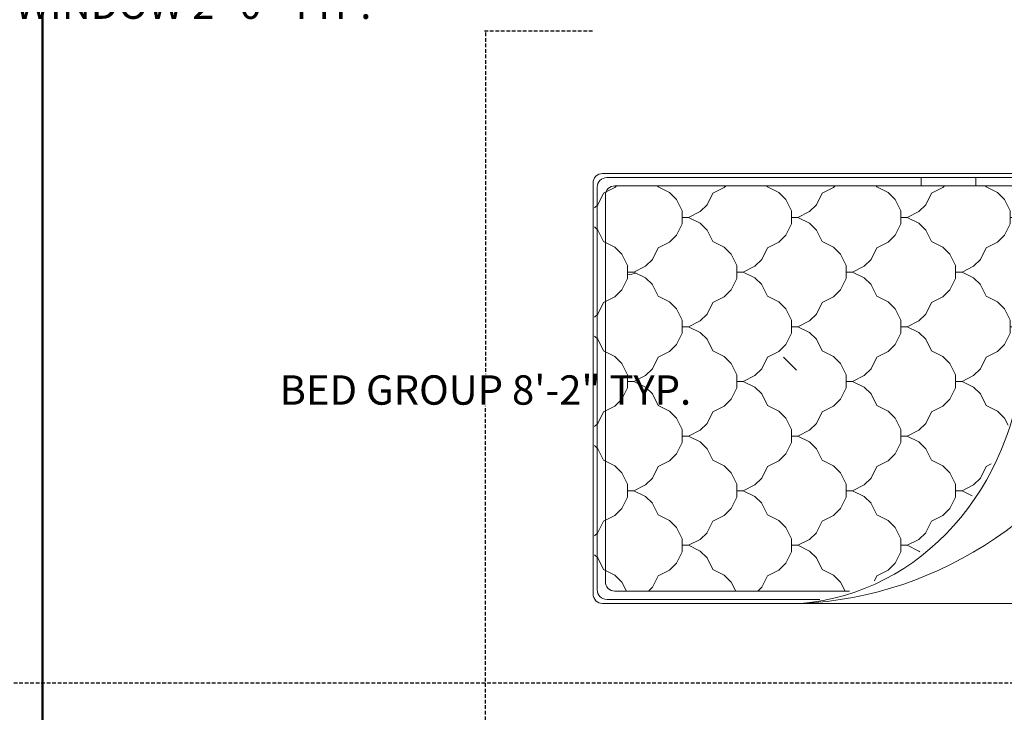
# Model space of a CAD drawing. Units: inches. Extents: x 513 to 1142, y 396 to 927.
# Tile 29 of 31: x 922 to 1056, y 770 to 865. Entities that reach past the tile are written whole.
import ezdxf

# ---------------------------------------------------------------- set-up
doc = ezdxf.new("R2010")
doc.units = ezdxf.units.IN
doc.header["$MEASUREMENT"] = 0
doc.linetypes.add('DASHED', pattern=[0.75, 0.5, -0.25])
for name, color, linetype, lineweight in [('A-ANNO-DIMS', 2, 'DASHED', 18), ('A-WALL', 7, 'Continuous', 50), ('furniture', 92, 'Continuous', 18)]:
    doc.layers.add(name, color=color, linetype=linetype, lineweight=lineweight)
doc.styles.get("Standard").update_dxf_attribs({"font": 'arial.ttf'})
doc.dimstyles.get("Standard").update_dxf_attribs({"dimtxt": 4, "dimasz": 0.18, "dimexe": 0.18, "dimexo": 0.0625, "dimgap": 0.09, "dimtad": 0, "dimtih": 1, "dimtoh": 1, "dimdec": 0, "dimrnd": 6, "dimzin": 0, "dimdsep": 46, "dimlunit": 3, "dimtxsty": 'Standard', "dimcen": 0.09, "dimadec": 0, "dimazin": 0, "dimtfac": 1, "dimtdec": 0, "dimtofl": 0, "dimtmove": 0, "dimatfit": 3, "dimfxl": 1, "dimtolj": 1, "dimtzin": 0, "dimarcsym": 0})

# ---------------------------------------------------------------- blocks, each defined once
blk = doc.blocks.new('A$C029D5C69')
for p, q in [((0.4164, 2.0693), (0.4164, 2.0066)), ((2.2315, 2.0693), (0.4164, 2.0693)), ((2.2315, 2.0066), (2.2315, 2.0693)), ((0, 1.606), (0, 2.0066)), ((0, 2.0066), (0.505, 2.0066)), ((0.4164, 2.0066), (2.2315, 2.0066)), ((0.505, 2.0066), (0.505, 1.606)), ((0.5252, 0.0351), (0.5252, 2.0066)), ((0.5403, 0.0502), (0.5403, 2.0066)), ((0.5706, 0.0805), (0.5706, 2.0066)), ((0.6869, 1.966), (0.6666, 2.0066)), ((0.7072, 2.0066), (0.6869, 1.966)), ((1.0902, 1.966), (1.0699, 2.0066)), ((1.1106, 2.0066), (1.0902, 1.966)), ((2.1114, 2.0087), (2.1114, 0.0351)), ((2.6479, 2.0066), (2.1429, 2.0066)), ((2.1429, 2.0066), (2.1429, 1.606)), ((2.6479, 1.606), (2.6479, 2.0066)), ((0.0151, 1.6211), (0.0151, 1.9915)), ((0.0151, 1.9915), (0.4899, 1.9915)), ((0.4899, 1.9915), (0.4899, 1.6211)), ((0.6869, 1.9425), (0.6869, 1.966)), ((0.6869, 1.9425), (0.6869, 1.966)), ((1.0902, 1.9425), (1.0902, 1.966)), ((1.0902, 1.9425), (1.0902, 1.966)), ((1.8954, 1.9865), (1.3081, 1.9865)), ((1.8954, 1.9713), (1.3339, 1.9713)), ((1.3849, 1.9713), (1.3656, 1.952)), ((1.3945, 1.9713), (1.3714, 1.9483)), ((1.4249, 1.945), (1.3986, 1.9713)), ((1.4288, 1.9507), (1.4081, 1.9713)), ((1.487, 1.9713), (1.4664, 1.9507)), ((1.4966, 1.9713), (1.4703, 1.945)), ((1.527, 1.945), (1.5007, 1.9713)), ((1.5309, 1.9507), (1.5102, 1.9713)), ((1.5891, 1.9713), (1.5685, 1.9507)), ((1.5987, 1.9713), (1.5724, 1.945)), ((1.6291, 1.945), (1.6028, 1.9713)), ((1.633, 1.9507), (1.6123, 1.9713)), ((1.6912, 1.9713), (1.6706, 1.9507)), ((1.7008, 1.9713), (1.6745, 1.945)), ((1.7312, 1.945), (1.7049, 1.9713)), ((1.7351, 1.9507), (1.7144, 1.9713)), ((1.7933, 1.9713), (1.7727, 1.9507)), ((1.8029, 1.9713), (1.7766, 1.945)), ((1.8333, 1.945), (1.807, 1.9713)), ((1.8372, 1.9507), (1.8165, 1.9713)), ((1.8954, 1.9713), (1.8748, 1.9507)), ((1.9043, 1.9707), (1.8787, 1.945)), ((1.9354, 1.945), (1.9114, 1.969)), ((2.6328, 1.9915), (2.158, 1.9915)), ((2.158, 1.9915), (2.158, 1.6211)), ((2.6328, 1.6211), (2.6328, 1.9915)), ((0.2689, 1.9609), (0.2689, 1.6764)), ((0.6634, 1.9425), (0.621, 1.9213)), ((0.6634, 1.9425), (0.621, 1.9213)), ((0.6869, 1.9425), (0.6634, 1.9425)), ((0.6869, 1.9425), (0.7104, 1.9425)), ((0.7528, 1.9213), (0.7104, 1.9425)), ((0.7528, 1.9213), (0.7104, 1.9425)), ((1.0668, 1.9425), (1.0244, 1.9213)), ((1.0668, 1.9425), (1.0244, 1.9213)), ((1.0902, 1.9425), (1.0668, 1.9425)), ((1.0902, 1.9425), (1.1137, 1.9425)), ((1.1561, 1.9213), (1.1137, 1.9425)), ((1.1561, 1.9213), (1.1137, 1.9425)), ((1.4249, 1.945), (1.4059, 1.926)), ((1.4288, 1.9394), (1.4116, 1.9222)), ((1.4476, 1.9507), (1.4288, 1.9507)), ((1.4288, 1.9393), (1.4476, 1.9393)), ((1.4476, 1.9507), (1.4664, 1.9507)), ((1.4664, 1.9393), (1.4476, 1.9393)), ((1.493, 1.9128), (1.4664, 1.9394)), ((1.4986, 1.9167), (1.4703, 1.945)), ((1.527, 1.945), (1.4986, 1.9167)), ((1.5309, 1.9394), (1.5043, 1.9128)), ((1.5497, 1.9507), (1.5309, 1.9507)), ((1.5309, 1.9393), (1.5497, 1.9393)), ((1.5497, 1.9507), (1.5685, 1.9507)), ((1.5685, 1.9393), (1.5497, 1.9393)), ((1.595, 1.9128), (1.5685, 1.9394)), ((1.6007, 1.9167), (1.5724, 1.945)), ((1.6291, 1.945), (1.6007, 1.9167)), ((1.633, 1.9394), (1.6064, 1.9128)), ((1.6518, 1.9507), (1.633, 1.9507)), ((1.633, 1.9393), (1.6518, 1.9393)), ((1.6518, 1.9507), (1.6706, 1.9507)), ((1.6706, 1.9393), (1.6518, 1.9393)), ((1.6971, 1.9128), (1.6706, 1.9394)), ((1.7028, 1.9167), (1.6745, 1.945)), ((1.7312, 1.945), (1.7028, 1.9167)), ((1.7351, 1.9394), (1.7085, 1.9128)), ((1.7539, 1.9507), (1.7351, 1.9507)), ((1.7351, 1.9393), (1.7539, 1.9393)), ((1.7539, 1.9507), (1.7727, 1.9507)), ((1.7727, 1.9393), (1.7539, 1.9393)), ((1.7992, 1.9128), (1.7727, 1.9394)), ((1.8049, 1.9167), (1.7766, 1.945)), ((1.8333, 1.945), (1.8049, 1.9167)), ((1.8372, 1.9394), (1.8106, 1.9128)), ((1.856, 1.9507), (1.8372, 1.9507)), ((1.8372, 1.9393), (1.856, 1.9393)), ((1.856, 1.9507), (1.8748, 1.9507)), ((1.8748, 1.9393), (1.856, 1.9393)), ((1.9013, 1.9128), (1.8748, 1.9394)), ((1.907, 1.9167), (1.8787, 1.945)), ((1.9354, 1.945), (1.907, 1.9167)), ((1.9393, 1.9394), (1.9127, 1.9128)), ((1.9393, 1.9393), (1.9404, 1.9393)), ((1.9414, 1.688), (1.9414, 1.931)), ((1.9565, 1.688), (1.9565, 1.931)), ((2.379, 1.9609), (2.379, 1.6764)), ((0.5955, 1.8958), (0.5743, 1.8534)), ((0.621, 1.9213), (0.5955, 1.8958)), ((0.7783, 1.8958), (0.7528, 1.9213)), ((0.7995, 1.8534), (0.7783, 1.8958)), ((0.9989, 1.8958), (0.9777, 1.8534)), ((1.0243, 1.9213), (0.9988, 1.8958)), ((1.1816, 1.8958), (1.1561, 1.9213)), ((1.2028, 1.8534), (1.1816, 1.8958)), ((1.493, 1.8752), (1.493, 1.9128)), ((1.5043, 1.8752), (1.5043, 1.9128)), ((1.595, 1.8752), (1.595, 1.9128)), ((1.6064, 1.8752), (1.6064, 1.9128)), ((1.6971, 1.8752), (1.6971, 1.9128)), ((1.7085, 1.8752), (1.7085, 1.9128)), ((1.7992, 1.8752), (1.7992, 1.9128)), ((1.8106, 1.8752), (1.8106, 1.9128)), ((1.9013, 1.8752), (1.9013, 1.9128)), ((1.9127, 1.8752), (1.9127, 1.9128)), ((0.5743, 1.8534), (0.5706, 1.8515)), ((0.5743, 1.8534), (0.5706, 1.8515)), ((0.8419, 1.8322), (0.7995, 1.8534)), ((0.8419, 1.8322), (0.7995, 1.8534)), ((0.9777, 1.8534), (0.9353, 1.8322)), ((0.9777, 1.8534), (0.9353, 1.8322)), ((1.2452, 1.8322), (1.2028, 1.8534)), ((1.2452, 1.8322), (1.2028, 1.8534)), ((1.493, 1.8752), (1.4867, 1.869)), ((1.4986, 1.8713), (1.4922, 1.8648)), ((1.527, 1.8429), (1.4986, 1.8713)), ((1.5309, 1.8486), (1.5043, 1.8752)), ((1.595, 1.8752), (1.5685, 1.8486)), ((1.6007, 1.8713), (1.5724, 1.8429)), ((1.6291, 1.8429), (1.6007, 1.8713)), ((1.633, 1.8486), (1.6064, 1.8752)), ((1.6971, 1.8752), (1.6706, 1.8486)), ((1.7028, 1.8713), (1.6745, 1.8429)), ((1.7312, 1.8429), (1.7028, 1.8713)), ((1.7351, 1.8486), (1.7085, 1.8752)), ((1.7992, 1.8752), (1.7727, 1.8486)), ((1.8049, 1.8713), (1.7766, 1.8429)), ((1.8333, 1.8429), (1.8049, 1.8713)), ((1.8372, 1.8486), (1.8106, 1.8752)), ((1.9013, 1.8752), (1.8748, 1.8486)), ((1.907, 1.8713), (1.8787, 1.8429)), ((1.9354, 1.8429), (1.907, 1.8713)), ((1.9393, 1.8486), (1.9127, 1.8752)), ((0.1267, 1.8186), (0.4111, 1.8186)), ((0.8674, 1.8067), (0.8419, 1.8322)), ((0.9352, 1.8322), (0.9097, 1.8067)), ((1.2707, 1.8067), (1.2452, 1.8322)), ((1.527, 1.8429), (1.5242, 1.8401)), ((1.5309, 1.8373), (1.5295, 1.8359)), ((1.5497, 1.8486), (1.5309, 1.8486)), ((1.5309, 1.8373), (1.5497, 1.8373)), ((1.5497, 1.8486), (1.5685, 1.8486)), ((1.5685, 1.8373), (1.5497, 1.8373)), ((1.595, 1.8107), (1.5685, 1.8373)), ((1.6007, 1.8146), (1.5724, 1.8429)), ((1.6291, 1.8429), (1.6007, 1.8146)), ((1.633, 1.8373), (1.6064, 1.8107)), ((1.6518, 1.8486), (1.633, 1.8486)), ((1.633, 1.8373), (1.6518, 1.8373)), ((1.6518, 1.8486), (1.6706, 1.8486)), ((1.6706, 1.8373), (1.6518, 1.8373)), ((1.6971, 1.8107), (1.6706, 1.8373)), ((1.7028, 1.8146), (1.6745, 1.8429)), ((1.7312, 1.8429), (1.7028, 1.8146)), ((1.7351, 1.8373), (1.7085, 1.8107)), ((1.7539, 1.8486), (1.7351, 1.8486)), ((1.7351, 1.8373), (1.7539, 1.8373)), ((1.7539, 1.8486), (1.7727, 1.8486)), ((1.7727, 1.8373), (1.7539, 1.8373)), ((1.7992, 1.8107), (1.7727, 1.8373)), ((1.8049, 1.8146), (1.7766, 1.8429)), ((1.8333, 1.8429), (1.8049, 1.8146)), ((1.8372, 1.8373), (1.8106, 1.8107)), ((1.856, 1.8486), (1.8372, 1.8486)), ((1.8372, 1.8373), (1.856, 1.8373)), ((1.856, 1.8486), (1.8748, 1.8486)), ((1.8748, 1.8373), (1.856, 1.8373)), ((1.9013, 1.8107), (1.8748, 1.8373)), ((1.907, 1.8146), (1.8787, 1.8429)), ((1.9354, 1.8429), (1.907, 1.8146)), ((1.9393, 1.8373), (1.9127, 1.8107)), ((1.9414, 1.8486), (1.9393, 1.8486)), ((1.9393, 1.8373), (1.9414, 1.8373)), ((2.2367, 1.8186), (2.5212, 1.8186)), ((0.8886, 1.7643), (0.8674, 1.8067)), ((0.9098, 1.8067), (0.8886, 1.7643)), ((1.2919, 1.7643), (1.2707, 1.8067)), ((1.595, 1.7806), (1.595, 1.8107)), ((1.6064, 1.7731), (1.6064, 1.8107)), ((1.6971, 1.7731), (1.6971, 1.8107)), ((1.7085, 1.7731), (1.7085, 1.8107)), ((1.7992, 1.7731), (1.7992, 1.8107)), ((1.8106, 1.7731), (1.8106, 1.8107)), ((1.9013, 1.7731), (1.9013, 1.8107)), ((1.9127, 1.7731), (1.9127, 1.8107)), ((0.8886, 1.7408), (0.8886, 1.7643)), ((1.2981, 1.7768), (1.2919, 1.7643)), ((1.2919, 1.7519), (1.2919, 1.7643)), ((1.633, 1.7465), (1.6064, 1.7731)), ((1.6518, 1.7465), (1.633, 1.7465)), ((1.6518, 1.7465), (1.6706, 1.7465)), ((1.6971, 1.7731), (1.6706, 1.7465)), ((1.7028, 1.7692), (1.6745, 1.7408)), ((1.7312, 1.7408), (1.7028, 1.7692)), ((1.7351, 1.7465), (1.7085, 1.7731)), ((1.7539, 1.7465), (1.7351, 1.7465)), ((1.7539, 1.7465), (1.7727, 1.7465)), ((1.7992, 1.7731), (1.7727, 1.7465)), ((1.8049, 1.7692), (1.7766, 1.7408)), ((1.8333, 1.7408), (1.8049, 1.7692)), ((1.8372, 1.7465), (1.8106, 1.7731)), ((1.856, 1.7465), (1.8372, 1.7465)), ((1.856, 1.7465), (1.8748, 1.7465)), ((1.9013, 1.7731), (1.8748, 1.7465)), ((1.907, 1.7692), (1.8787, 1.7408)), ((1.9354, 1.7408), (1.907, 1.7692)), ((1.9393, 1.7465), (1.9127, 1.7731)), ((1.9414, 1.7465), (1.9393, 1.7465)), ((0.8227, 1.7196), (0.7972, 1.6941)), ((0.8651, 1.7408), (0.8227, 1.7196)), ((0.8651, 1.7408), (0.8227, 1.7196)), ((0.912, 1.7408), (0.8651, 1.7408)), ((0.9544, 1.7196), (0.912, 1.7408)), ((0.9544, 1.7196), (0.912, 1.7408)), ((0.98, 1.6941), (0.9545, 1.7196)), ((1.226, 1.7196), (1.2005, 1.6941)), ((1.2684, 1.7408), (1.226, 1.7196)), ((1.2684, 1.7408), (1.226, 1.7196)), ((1.2885, 1.7408), (1.2684, 1.7408)), ((1.6443, 1.7352), (1.6518, 1.7352)), ((1.6706, 1.7352), (1.6518, 1.7352)), ((1.6971, 1.7086), (1.6706, 1.7352)), ((1.7028, 1.7125), (1.6745, 1.7408)), ((1.6971, 1.682), (1.6971, 1.7086)), ((1.7312, 1.7408), (1.7028, 1.7125)), ((1.7351, 1.7352), (1.7085, 1.7086)), ((1.7085, 1.671), (1.7085, 1.7086)), ((1.7351, 1.7352), (1.7539, 1.7352)), ((1.7727, 1.7352), (1.7539, 1.7352)), ((1.7992, 1.7086), (1.7727, 1.7352)), ((1.8049, 1.7125), (1.7766, 1.7408)), ((1.7992, 1.671), (1.7992, 1.7086)), ((1.8333, 1.7408), (1.8049, 1.7125)), ((1.8372, 1.7352), (1.8106, 1.7086)), ((1.8106, 1.671), (1.8106, 1.7086)), ((1.8372, 1.7352), (1.856, 1.7352)), ((1.8748, 1.7352), (1.856, 1.7352)), ((1.9013, 1.7086), (1.8748, 1.7352)), ((1.907, 1.7125), (1.8787, 1.7408)), ((1.9013, 1.671), (1.9013, 1.7086)), ((1.9354, 1.7408), (1.907, 1.7125)), ((1.9393, 1.7352), (1.9127, 1.7086)), ((1.9127, 1.671), (1.9127, 1.7086)), ((1.9393, 1.7352), (1.9414, 1.7352)), ((0.5766, 1.6941), (0.5706, 1.7002)), ((0.5978, 1.6517), (0.5766, 1.6941)), ((0.7972, 1.6941), (0.776, 1.6517)), ((1.0011, 1.6517), (0.9799, 1.6941)), ((1.2005, 1.6941), (1.1793, 1.6517)), ((1.7318, 1.6477), (1.7085, 1.671)), ((1.7992, 1.671), (1.7759, 1.6477)), ((1.8339, 1.6477), (1.8106, 1.671)), ((1.9013, 1.671), (1.878, 1.6477)), ((1.926, 1.6577), (1.9127, 1.671)), ((2.5551, 1.6275), (2.5551, 1.696)), ((0.6402, 1.6305), (0.5978, 1.6517)), ((0.6402, 1.6305), (0.5978, 1.6517)), ((0.776, 1.6517), (0.7336, 1.6305)), ((0.776, 1.6517), (0.7336, 1.6305)), ((1.0435, 1.6305), (1.0011, 1.6517)), ((1.0435, 1.6305), (1.0011, 1.6517)), ((1.1793, 1.6517), (1.1369, 1.6305)), ((1.1793, 1.6517), (1.1369, 1.6305)), ((1.8961, 1.6477), (1.7289, 1.6477)), ((1.8049, 1.6671), (1.7855, 1.6477)), ((1.8244, 1.6477), (1.8049, 1.6671)), ((1.907, 1.6671), (1.8876, 1.6477)), ((1.9202, 1.6539), (1.907, 1.6671)), ((0.505, 1.606), (0, 1.606)), ((0.4899, 1.6211), (0.0151, 1.6211)), ((0.6657, 1.605), (0.6402, 1.6305)), ((0.6869, 1.5626), (0.6657, 1.605)), ((0.7081, 1.605), (0.6869, 1.5626)), ((0.7336, 1.6305), (0.7081, 1.605)), ((1.0691, 1.605), (1.0436, 1.6305)), ((1.0902, 1.5626), (1.069, 1.605)), ((1.1114, 1.605), (1.0902, 1.5626)), ((1.1369, 1.6305), (1.1114, 1.605)), ((1.8961, 1.6325), (1.7422, 1.6325)), ((2.1429, 1.606), (2.6479, 1.606)), ((2.158, 1.6211), (2.6328, 1.6211)), ((0.6869, 1.5392), (0.6869, 1.5626)), ((0.6869, 1.5392), (0.6869, 1.5626)), ((1.0902, 1.5392), (1.0902, 1.5626)), ((1.0902, 1.5392), (1.0902, 1.5626)), ((0.6634, 1.5391), (0.621, 1.5179)), ((0.6634, 1.5391), (0.621, 1.5179)), ((0.6869, 1.5392), (0.6634, 1.5392)), ((0.6869, 1.5392), (0.7104, 1.5392)), ((0.7528, 1.5179), (0.7104, 1.5391)), ((0.7528, 1.5179), (0.7104, 1.5391)), ((1.0668, 1.5391), (1.0244, 1.5179)), ((1.0668, 1.5391), (1.0244, 1.5179)), ((1.0902, 1.5392), (1.0668, 1.5392)), ((1.0902, 1.5392), (1.1137, 1.5392)), ((1.1561, 1.5179), (1.1137, 1.5391)), ((1.1561, 1.5179), (1.1137, 1.5391)), ((1.4534, 1.5308), (1.4277, 1.5179)), ((1.4534, 1.5308), (1.4277, 1.5179)), ((0.5955, 1.4925), (0.5743, 1.4501)), ((0.621, 1.5179), (0.5955, 1.4924)), ((0.7783, 1.4924), (0.7528, 1.5179)), ((0.7995, 1.4501), (0.7783, 1.4925)), ((0.9989, 1.4925), (0.9777, 1.4501)), ((1.0243, 1.5179), (0.9988, 1.4924)), ((1.1816, 1.4924), (1.1561, 1.5179)), ((1.2028, 1.4501), (1.1816, 1.4925)), ((1.4022, 1.4925), (1.381, 1.4501)), ((1.4277, 1.5179), (1.4022, 1.4924)), ((1.6062, 1.4501), (1.5966, 1.4692)), ((0.5743, 1.45), (0.5706, 1.4481)), ((0.5743, 1.45), (0.5706, 1.4481)), ((0.8419, 1.4288), (0.7995, 1.45)), ((0.8419, 1.4288), (0.7995, 1.45)), ((0.8674, 1.4033), (0.8419, 1.4288)), ((0.9352, 1.4288), (0.9097, 1.4033)), ((0.9777, 1.45), (0.9353, 1.4288)), ((0.9777, 1.45), (0.9353, 1.4288)), ((1.2452, 1.4288), (1.2028, 1.45)), ((1.2452, 1.4288), (1.2028, 1.45)), ((1.2707, 1.4033), (1.2452, 1.4288)), ((1.3386, 1.4288), (1.3131, 1.4033)), ((1.381, 1.45), (1.3386, 1.4288)), ((1.381, 1.45), (1.3386, 1.4288)), ((1.6486, 1.4288), (1.6062, 1.45)), ((1.6486, 1.4288), (1.6062, 1.45)), ((1.6741, 1.4033), (1.6486, 1.4288)), ((0.5403, 1.4117), (0.5706, 1.4117)), ((0.8886, 1.361), (0.8674, 1.4034)), ((0.9098, 1.4034), (0.8886, 1.361)), ((1.2919, 1.361), (1.2707, 1.4034)), ((1.3131, 1.4034), (1.2919, 1.361)), ((1.6953, 1.361), (1.6741, 1.4034)), ((1.714, 1.3984), (1.6953, 1.361)), ((0.8886, 1.3375), (0.8886, 1.3609)), ((1.2919, 1.3375), (1.2919, 1.3609)), ((1.6953, 1.3375), (1.6953, 1.3609)), ((0.8227, 1.3163), (0.7972, 1.2908)), ((0.8651, 1.3374), (0.8227, 1.3162)), ((0.8651, 1.3374), (0.8227, 1.3162)), ((0.912, 1.3375), (0.8651, 1.3375)), ((0.9544, 1.3162), (0.912, 1.3374)), ((0.9544, 1.3162), (0.912, 1.3374)), ((0.98, 1.2908), (0.9545, 1.3163)), ((1.226, 1.3163), (1.2005, 1.2908)), ((1.2684, 1.3374), (1.226, 1.3162)), ((1.2684, 1.3374), (1.226, 1.3162)), ((1.3154, 1.3375), (1.2684, 1.3375)), ((1.3578, 1.3162), (1.3154, 1.3374)), ((1.3578, 1.3162), (1.3154, 1.3374)), ((1.3833, 1.2908), (1.3578, 1.3163)), ((1.6294, 1.3163), (1.6039, 1.2908)), ((1.6718, 1.3374), (1.6294, 1.3162)), ((1.6718, 1.3374), (1.6294, 1.3162)), ((1.7187, 1.3375), (1.6718, 1.3375)), ((1.7611, 1.3162), (1.7187, 1.3374)), ((1.7611, 1.3162), (1.7187, 1.3374)), ((1.7867, 1.2908), (1.7611, 1.3163)), ((0.5766, 1.2908), (0.5706, 1.2968)), ((0.5978, 1.2484), (0.5766, 1.2908)), ((0.7972, 1.2908), (0.776, 1.2484)), ((1.0011, 1.2484), (0.9799, 1.2908)), ((1.2005, 1.2908), (1.1793, 1.2484)), ((1.4045, 1.2484), (1.3833, 1.2908)), ((1.6039, 1.2908), (1.5827, 1.2484)), ((1.8078, 1.2484), (1.7866, 1.2908)), ((0.6402, 1.2271), (0.5978, 1.2483)), ((0.6402, 1.2271), (0.5978, 1.2483)), ((0.776, 1.2483), (0.7336, 1.2271)), ((0.776, 1.2483), (0.7336, 1.2271)), ((1.0435, 1.2271), (1.0011, 1.2483)), ((1.0435, 1.2271), (1.0011, 1.2483)), ((1.1793, 1.2483), (1.1369, 1.2271)), ((1.1793, 1.2483), (1.1369, 1.2271)), ((1.4469, 1.2271), (1.4045, 1.2483)), ((1.4469, 1.2271), (1.4045, 1.2483)), ((1.5827, 1.2483), (1.5403, 1.2271)), ((1.5827, 1.2483), (1.5403, 1.2271)), ((1.8502, 1.2271), (1.8078, 1.2483)), ((1.8502, 1.2271), (1.8078, 1.2483)), ((0.5403, 1.21), (0.5706, 1.21)), ((0.6657, 1.2017), (0.6402, 1.2272)), ((0.6869, 1.1593), (0.6657, 1.2017)), ((0.7081, 1.2017), (0.6869, 1.1593)), ((0.7336, 1.2272), (0.7081, 1.2017)), ((1.0691, 1.2017), (1.0436, 1.2272)), ((1.0902, 1.1593), (1.069, 1.2017)), ((1.1114, 1.2017), (1.0902, 1.1593)), ((1.1369, 1.2272), (1.1114, 1.2017)), ((1.4724, 1.2017), (1.4469, 1.2272)), ((1.4936, 1.1593), (1.4724, 1.2017)), ((1.5148, 1.2017), (1.4936, 1.1593)), ((1.5403, 1.2272), (1.5148, 1.2017)), ((1.8758, 1.2017), (1.8503, 1.2272)), ((1.8969, 1.1593), (1.8757, 1.2017)), ((1.9181, 1.2017), (1.8969, 1.1593)), ((1.9215, 1.2051), (1.9181, 1.2017)), ((0.6634, 1.1358), (0.621, 1.1146)), ((0.6634, 1.1358), (0.621, 1.1146)), ((0.6869, 1.1358), (0.6634, 1.1358)), ((0.6869, 1.1358), (0.6869, 1.1593)), ((0.6869, 1.1358), (0.6869, 1.1593)), ((0.6869, 1.1358), (0.7104, 1.1358)), ((0.7528, 1.1146), (0.7104, 1.1358)), ((0.7528, 1.1146), (0.7104, 1.1358)), ((1.0668, 1.1358), (1.0244, 1.1146)), ((1.0668, 1.1358), (1.0244, 1.1146)), ((1.0902, 1.1358), (1.0668, 1.1358)), ((1.0902, 1.1358), (1.0902, 1.1593)), ((1.0902, 1.1358), (1.0902, 1.1593)), ((1.0902, 1.1358), (1.1137, 1.1358)), ((1.1561, 1.1146), (1.1137, 1.1358)), ((1.1561, 1.1146), (1.1137, 1.1358)), ((1.4701, 1.1358), (1.4277, 1.1146)), ((1.4701, 1.1358), (1.4277, 1.1146)), ((1.4936, 1.1358), (1.4701, 1.1358)), ((1.4936, 1.1358), (1.4936, 1.1593)), ((1.4936, 1.1358), (1.4936, 1.1593)), ((1.4936, 1.1358), (1.5171, 1.1358)), ((1.5595, 1.1146), (1.5171, 1.1358)), ((1.5595, 1.1146), (1.5171, 1.1358)), ((1.8735, 1.1358), (1.8311, 1.1146)), ((1.8735, 1.1358), (1.8311, 1.1146)), ((1.8969, 1.1358), (1.8735, 1.1358)), ((1.8969, 1.1358), (1.8969, 1.1593)), ((1.8969, 1.1358), (1.8969, 1.1593)), ((1.8969, 1.1358), (1.9204, 1.1358)), ((1.9628, 1.1146), (1.9204, 1.1358)), ((1.9628, 1.1146), (1.9204, 1.1358)), ((0.621, 1.1146), (0.5955, 1.0891)), ((0.7783, 1.0891), (0.7528, 1.1146)), ((1.0243, 1.1146), (0.9988, 1.0891)), ((1.1816, 1.0891), (1.1561, 1.1146)), ((1.4277, 1.1146), (1.4022, 1.0891)), ((1.585, 1.0891), (1.5595, 1.1146)), ((1.831, 1.1146), (1.8055, 1.0891)), ((1.9883, 1.0891), (1.9628, 1.1146)), ((0.5955, 1.0891), (0.5743, 1.0467)), ((0.7995, 1.0467), (0.7783, 1.0891)), ((0.9989, 1.0891), (0.9777, 1.0467)), ((1.2028, 1.0467), (1.1816, 1.0891)), ((1.4022, 1.0891), (1.381, 1.0467)), ((1.6062, 1.0467), (1.585, 1.0891)), ((1.8056, 1.0891), (1.7844, 1.0467)), ((2.0095, 1.0467), (1.9883, 1.0891)), ((0.5743, 1.0467), (0.5706, 1.0448)), ((0.5743, 1.0467), (0.5706, 1.0448)), ((0.8419, 1.0255), (0.7995, 1.0467)), ((0.8419, 1.0255), (0.7995, 1.0467)), ((0.8674, 1), (0.8419, 1.0255)), ((0.9352, 1.0255), (0.9097, 1)), ((0.9777, 1.0467), (0.9353, 1.0255)), ((0.9777, 1.0467), (0.9353, 1.0255)), ((1.2452, 1.0255), (1.2028, 1.0467)), ((1.2452, 1.0255), (1.2028, 1.0467)), ((1.2707, 1), (1.2452, 1.0255)), ((1.3386, 1.0255), (1.3131, 1)), ((1.381, 1.0467), (1.3386, 1.0255)), ((1.381, 1.0467), (1.3386, 1.0255)), ((1.6486, 1.0255), (1.6062, 1.0467)), ((1.6486, 1.0255), (1.6062, 1.0467)), ((1.6741, 1), (1.6486, 1.0255)), ((1.7419, 1.0255), (1.7164, 1)), ((1.7844, 1.0467), (1.742, 1.0255)), ((1.7844, 1.0467), (1.742, 1.0255)), ((2.0276, 1.0376), (2.0095, 1.0467)), ((2.0276, 1.0376), (2.0095, 1.0467)), ((0.8886, 0.9576), (0.8674, 1)), ((0.9098, 1), (0.8886, 0.9576)), ((1.2919, 0.9576), (1.2707, 1)), ((1.3131, 1), (1.2919, 0.9576)), ((1.6953, 0.9576), (1.6741, 1)), ((1.7165, 1), (1.6953, 0.9576)), ((0.8886, 0.9341), (0.8886, 0.9576)), ((1.2919, 0.9341), (1.2919, 0.9576)), ((1.6953, 0.9341), (1.6953, 0.9576)), ((2.066, 0.9457), (2.066, 0.0805)), ((0.8227, 0.9129), (0.7972, 0.8874)), ((0.8651, 0.9341), (0.8227, 0.9129)), ((0.8651, 0.9341), (0.8227, 0.9129)), ((0.912, 0.9341), (0.8651, 0.9341)), ((0.9544, 0.9129), (0.912, 0.9341)), ((0.9544, 0.9129), (0.912, 0.9341)), ((0.98, 0.8874), (0.9545, 0.9129)), ((1.226, 0.9129), (1.2005, 0.8874)), ((1.2684, 0.9341), (1.226, 0.9129)), ((1.2684, 0.9341), (1.226, 0.9129)), ((1.3154, 0.9341), (1.2684, 0.9341)), ((1.3578, 0.9129), (1.3154, 0.9341)), ((1.3578, 0.9129), (1.3154, 0.9341)), ((1.3833, 0.8874), (1.3578, 0.9129)), ((1.6294, 0.9129), (1.6039, 0.8874)), ((1.6718, 0.9341), (1.6294, 0.9129)), ((1.6718, 0.9341), (1.6294, 0.9129)), ((1.7187, 0.9341), (1.6718, 0.9341)), ((1.7611, 0.9129), (1.7187, 0.9341)), ((1.7611, 0.9129), (1.7187, 0.9341)), ((1.7867, 0.8874), (1.7611, 0.9129)), ((2.0327, 0.9129), (2.0072, 0.8874)), ((2.066, 0.9295), (2.0327, 0.9129)), ((2.066, 0.9295), (2.0327, 0.9129)), ((0.5766, 0.8874), (0.5706, 0.8935)), ((0.5978, 0.845), (0.5766, 0.8874)), ((0.7972, 0.8874), (0.776, 0.845)), ((1.0011, 0.845), (0.9799, 0.8874)), ((1.2005, 0.8874), (1.1793, 0.845)), ((1.4045, 0.845), (1.3833, 0.8874)), ((1.6039, 0.8874), (1.5827, 0.845)), ((1.8078, 0.845), (1.7866, 0.8874)), ((2.0072, 0.8874), (1.986, 0.845)), ((0.6402, 0.8238), (0.5978, 0.845)), ((0.6402, 0.8238), (0.5978, 0.845)), ((0.776, 0.845), (0.7336, 0.8238)), ((0.776, 0.845), (0.7336, 0.8238)), ((1.0435, 0.8238), (1.0011, 0.845)), ((1.0435, 0.8238), (1.0011, 0.845)), ((1.1793, 0.845), (1.1369, 0.8238)), ((1.1793, 0.845), (1.1369, 0.8238)), ((1.4469, 0.8238), (1.4045, 0.845)), ((1.4469, 0.8238), (1.4045, 0.845)), ((1.5827, 0.845), (1.5403, 0.8238)), ((1.5827, 0.845), (1.5403, 0.8238)), ((1.8502, 0.8238), (1.8078, 0.845)), ((1.8502, 0.8238), (1.8078, 0.845)), ((1.986, 0.845), (1.9436, 0.8238)), ((1.986, 0.845), (1.9436, 0.8238)), ((2.0962, 0.8369), (2.0962, 0.0502)), ((0.6657, 0.7983), (0.6402, 0.8238)), ((0.7336, 0.8238), (0.7081, 0.7983)), ((1.0691, 0.7983), (1.0436, 0.8238)), ((1.1369, 0.8238), (1.1114, 0.7983)), ((1.4724, 0.7983), (1.4469, 0.8238)), ((1.5403, 0.8238), (1.5148, 0.7983)), ((1.8758, 0.7983), (1.8503, 0.8238)), ((1.9436, 0.8238), (1.9181, 0.7983)), ((0.6869, 0.7559), (0.6657, 0.7983)), ((0.7081, 0.7983), (0.6869, 0.7559)), ((1.0902, 0.7559), (1.069, 0.7983)), ((1.1114, 0.7983), (1.0902, 0.7559)), ((1.4936, 0.7559), (1.4724, 0.7983)), ((1.5148, 0.7983), (1.4936, 0.7559)), ((1.8969, 0.7559), (1.8757, 0.7983)), ((1.9181, 0.7983), (1.8969, 0.7559)), ((0.6634, 0.7324), (0.621, 0.7112)), ((0.6634, 0.7324), (0.621, 0.7112)), ((0.6869, 0.7325), (0.6634, 0.7325)), ((0.6869, 0.7325), (0.6869, 0.7559)), ((0.6869, 0.7325), (0.6869, 0.7559)), ((0.6869, 0.7325), (0.7104, 0.7325)), ((0.7528, 0.7112), (0.7104, 0.7324)), ((0.7528, 0.7112), (0.7104, 0.7324)), ((1.0668, 0.7324), (1.0244, 0.7112)), ((1.0668, 0.7324), (1.0244, 0.7112)), ((1.0902, 0.7325), (1.0668, 0.7325)), ((1.0902, 0.7325), (1.0902, 0.7559)), ((1.0902, 0.7325), (1.0902, 0.7559)), ((1.0902, 0.7325), (1.1137, 0.7325)), ((1.1561, 0.7112), (1.1137, 0.7324)), ((1.1561, 0.7112), (1.1137, 0.7324)), ((1.2024, 0.7028), (1.2503, 0.7507)), ((1.4701, 0.7324), (1.4277, 0.7112)), ((1.4701, 0.7324), (1.4277, 0.7112)), ((1.4936, 0.7325), (1.4701, 0.7325)), ((1.4936, 0.7325), (1.4936, 0.7559)), ((1.4936, 0.7325), (1.4936, 0.7559)), ((1.4936, 0.7325), (1.5171, 0.7325)), ((1.5595, 0.7112), (1.5171, 0.7324)), ((1.5595, 0.7112), (1.5171, 0.7324)), ((1.8735, 0.7324), (1.8311, 0.7112)), ((1.8735, 0.7324), (1.8311, 0.7112)), ((1.8969, 0.7325), (1.8735, 0.7325)), ((1.8969, 0.7325), (1.8969, 0.7559)), ((1.8969, 0.7325), (1.8969, 0.7559)), ((1.8969, 0.7325), (1.9204, 0.7325)), ((1.9628, 0.7112), (1.9204, 0.7324)), ((1.9628, 0.7112), (1.9204, 0.7324)), ((0.621, 0.7113), (0.5955, 0.6858)), ((0.7783, 0.6858), (0.7528, 0.7113)), ((1.0243, 0.7113), (0.9988, 0.6858)), ((1.1816, 0.6858), (1.1561, 0.7113)), ((1.4277, 0.7113), (1.4022, 0.6858)), ((1.585, 0.6858), (1.5595, 0.7113)), ((1.831, 0.7113), (1.8055, 0.6858)), ((1.9883, 0.6858), (1.9628, 0.7113)), ((0.5955, 0.6858), (0.5743, 0.6434)), ((0.7995, 0.6434), (0.7783, 0.6858)), ((0.9989, 0.6858), (0.9777, 0.6434)), ((1.2028, 0.6434), (1.1816, 0.6858)), ((1.4022, 0.6858), (1.381, 0.6434)), ((1.6062, 0.6434), (1.585, 0.6858)), ((1.8056, 0.6858), (1.7844, 0.6434)), ((2.0095, 0.6434), (1.9883, 0.6858)), ((0.5743, 0.6433), (0.5706, 0.6414)), ((0.5743, 0.6433), (0.5706, 0.6414)), ((0.8419, 0.6221), (0.7995, 0.6433)), ((0.8419, 0.6221), (0.7995, 0.6433)), ((0.8674, 0.5967), (0.8419, 0.6222)), ((0.9352, 0.6222), (0.9097, 0.5967)), ((0.9777, 0.6433), (0.9353, 0.6221)), ((0.9777, 0.6433), (0.9353, 0.6221)), ((1.2452, 0.6221), (1.2028, 0.6433)), ((1.2452, 0.6221), (1.2028, 0.6433)), ((1.2707, 0.5967), (1.2452, 0.6222)), ((1.3386, 0.6222), (1.3131, 0.5967)), ((1.381, 0.6433), (1.3386, 0.6221)), ((1.381, 0.6433), (1.3386, 0.6221)), ((1.6486, 0.6221), (1.6062, 0.6433)), ((1.6486, 0.6221), (1.6062, 0.6433)), ((1.6741, 0.5967), (1.6486, 0.6222)), ((1.7419, 0.6222), (1.7164, 0.5967)), ((1.7844, 0.6433), (1.742, 0.6221)), ((1.7844, 0.6433), (1.742, 0.6221)), ((2.0519, 0.6221), (2.0095, 0.6433)), ((2.0519, 0.6221), (2.0095, 0.6433)), ((2.066, 0.6081), (2.0519, 0.6222)), ((0.8886, 0.5543), (0.8674, 0.5967)), ((0.9098, 0.5967), (0.8886, 0.5543)), ((1.2919, 0.5543), (1.2707, 0.5967)), ((1.3131, 0.5967), (1.2919, 0.5543)), ((1.6953, 0.5543), (1.6741, 0.5967)), ((1.7165, 0.5967), (1.6953, 0.5543)), ((0.8886, 0.5308), (0.8886, 0.5543)), ((1.2919, 0.5308), (1.2919, 0.5543)), ((1.6953, 0.5308), (1.6953, 0.5543)), ((0.8227, 0.5096), (0.7972, 0.4841)), ((0.8651, 0.5308), (0.8227, 0.5096)), ((0.8651, 0.5308), (0.8227, 0.5096)), ((0.912, 0.5308), (0.8651, 0.5308)), ((0.9544, 0.5096), (0.912, 0.5308)), ((0.9544, 0.5096), (0.912, 0.5308)), ((0.98, 0.4841), (0.9545, 0.5096)), ((1.226, 0.5096), (1.2005, 0.4841)), ((1.2684, 0.5308), (1.226, 0.5096)), ((1.2684, 0.5308), (1.226, 0.5096)), ((1.3154, 0.5308), (1.2684, 0.5308)), ((1.3578, 0.5096), (1.3154, 0.5308)), ((1.3578, 0.5096), (1.3154, 0.5308)), ((1.3833, 0.4841), (1.3578, 0.5096)), ((1.6294, 0.5096), (1.6039, 0.4841)), ((1.6718, 0.5308), (1.6294, 0.5096)), ((1.6718, 0.5308), (1.6294, 0.5096)), ((1.7187, 0.5308), (1.6718, 0.5308)), ((1.7611, 0.5096), (1.7187, 0.5308)), ((1.7611, 0.5096), (1.7187, 0.5308)), ((1.7867, 0.4841), (1.7611, 0.5096)), ((2.0327, 0.5096), (2.0072, 0.4841)), ((2.066, 0.5262), (2.0327, 0.5096)), ((2.066, 0.5262), (2.0327, 0.5096)), ((0.5766, 0.4841), (0.5706, 0.4901)), ((0.5978, 0.4417), (0.5766, 0.4841)), ((0.7972, 0.4841), (0.776, 0.4417)), ((1.0011, 0.4417), (0.9799, 0.4841)), ((1.2005, 0.4841), (1.1793, 0.4417)), ((1.4045, 0.4417), (1.3833, 0.4841)), ((1.6039, 0.4841), (1.5827, 0.4417)), ((1.8078, 0.4417), (1.7866, 0.4841)), ((2.0072, 0.4841), (1.986, 0.4417)), ((0.6402, 0.4205), (0.5978, 0.4417)), ((0.6402, 0.4205), (0.5978, 0.4417)), ((0.776, 0.4417), (0.7336, 0.4205)), ((0.776, 0.4417), (0.7336, 0.4205)), ((1.0435, 0.4205), (1.0011, 0.4417)), ((1.0435, 0.4205), (1.0011, 0.4417)), ((1.1793, 0.4417), (1.1369, 0.4205)), ((1.1793, 0.4417), (1.1369, 0.4205)), ((1.4469, 0.4205), (1.4045, 0.4417)), ((1.4469, 0.4205), (1.4045, 0.4417)), ((1.5827, 0.4417), (1.5403, 0.4205)), ((1.5827, 0.4417), (1.5403, 0.4205)), ((1.8502, 0.4205), (1.8078, 0.4417)), ((1.8502, 0.4205), (1.8078, 0.4417)), ((1.986, 0.4417), (1.9436, 0.4205)), ((1.986, 0.4417), (1.9436, 0.4205)), ((0.6657, 0.395), (0.6402, 0.4205)), ((0.7336, 0.4205), (0.7081, 0.395)), ((1.0691, 0.395), (1.0436, 0.4205)), ((1.1369, 0.4205), (1.1114, 0.395)), ((1.4724, 0.395), (1.4469, 0.4205)), ((1.5403, 0.4205), (1.5148, 0.395)), ((1.8758, 0.395), (1.8503, 0.4205)), ((1.9436, 0.4205), (1.9181, 0.395)), ((0.6869, 0.3526), (0.6657, 0.395)), ((0.7081, 0.395), (0.6869, 0.3526)), ((1.0902, 0.3526), (1.069, 0.395)), ((1.1114, 0.395), (1.0902, 0.3526)), ((1.4936, 0.3526), (1.4724, 0.395)), ((1.5148, 0.395), (1.4936, 0.3526)), ((1.8969, 0.3526), (1.8757, 0.395)), ((1.9181, 0.395), (1.8969, 0.3526)), ((0.6634, 0.3291), (0.621, 0.3079)), ((0.6634, 0.3291), (0.621, 0.3079)), ((0.6869, 0.3291), (0.6634, 0.3291)), ((0.6869, 0.3291), (0.6869, 0.3526)), ((0.6869, 0.3291), (0.6869, 0.3526)), ((0.6869, 0.3291), (0.7104, 0.3291)), ((0.7528, 0.3079), (0.7104, 0.3291)), ((0.7528, 0.3079), (0.7104, 0.3291)), ((1.0668, 0.3291), (1.0244, 0.3079)), ((1.0668, 0.3291), (1.0244, 0.3079)), ((1.0902, 0.3291), (1.0668, 0.3291)), ((1.0902, 0.3291), (1.0902, 0.3526)), ((1.0902, 0.3291), (1.0902, 0.3526)), ((1.0902, 0.3291), (1.1137, 0.3291)), ((1.1561, 0.3079), (1.1137, 0.3291)), ((1.1561, 0.3079), (1.1137, 0.3291)), ((1.4701, 0.3291), (1.4277, 0.3079)), ((1.4701, 0.3291), (1.4277, 0.3079)), ((1.4936, 0.3291), (1.4701, 0.3291)), ((1.4936, 0.3291), (1.4936, 0.3526)), ((1.4936, 0.3291), (1.4936, 0.3526)), ((1.4936, 0.3291), (1.5171, 0.3291)), ((1.5595, 0.3079), (1.5171, 0.3291)), ((1.5595, 0.3079), (1.5171, 0.3291)), ((1.8735, 0.3291), (1.8311, 0.3079)), ((1.8735, 0.3291), (1.8311, 0.3079)), ((1.8969, 0.3291), (1.8735, 0.3291)), ((1.8969, 0.3291), (1.8969, 0.3526)), ((1.8969, 0.3291), (1.8969, 0.3526)), ((1.8969, 0.3291), (1.9204, 0.3291)), ((1.9628, 0.3079), (1.9204, 0.3291)), ((1.9628, 0.3079), (1.9204, 0.3291)), ((0.621, 0.3079), (0.5955, 0.2824)), ((0.7783, 0.2824), (0.7528, 0.3079)), ((1.0243, 0.3079), (0.9988, 0.2824)), ((1.1816, 0.2824), (1.1561, 0.3079)), ((1.4277, 0.3079), (1.4022, 0.2824)), ((1.585, 0.2824), (1.5595, 0.3079)), ((1.831, 0.3079), (1.8055, 0.2824)), ((1.9883, 0.2824), (1.9628, 0.3079)), ((0.5955, 0.2824), (0.5743, 0.24)), ((0.7995, 0.24), (0.7783, 0.2824)), ((0.9989, 0.2824), (0.9777, 0.24)), ((1.2028, 0.24), (1.1816, 0.2824)), ((1.4022, 0.2824), (1.381, 0.24)), ((1.6062, 0.24), (1.585, 0.2824)), ((1.8056, 0.2824), (1.7844, 0.24)), ((2.0095, 0.24), (1.9883, 0.2824)), ((0.5743, 0.24), (0.5706, 0.2381)), ((0.5743, 0.24), (0.5706, 0.2381)), ((0.8419, 0.2188), (0.7995, 0.24)), ((0.8419, 0.2188), (0.7995, 0.24)), ((0.8674, 0.1933), (0.8419, 0.2188)), ((0.9352, 0.2188), (0.9097, 0.1933)), ((0.9777, 0.24), (0.9353, 0.2188)), ((0.9777, 0.24), (0.9353, 0.2188)), ((1.2452, 0.2188), (1.2028, 0.24)), ((1.2452, 0.2188), (1.2028, 0.24)), ((1.2707, 0.1933), (1.2452, 0.2188)), ((1.3386, 0.2188), (1.3131, 0.1933)), ((1.381, 0.24), (1.3386, 0.2188)), ((1.381, 0.24), (1.3386, 0.2188)), ((1.6486, 0.2188), (1.6062, 0.24)), ((1.6486, 0.2188), (1.6062, 0.24)), ((1.6741, 0.1933), (1.6486, 0.2188)), ((1.7419, 0.2188), (1.7164, 0.1933)), ((1.7844, 0.24), (1.742, 0.2188)), ((1.7844, 0.24), (1.742, 0.2188)), ((2.0519, 0.2188), (2.0095, 0.24)), ((2.0519, 0.2188), (2.0095, 0.24)), ((2.066, 0.2047), (2.0519, 0.2188)), ((0.8886, 0.1509), (0.8674, 0.1933)), ((0.9098, 0.1933), (0.8886, 0.1509)), ((1.2919, 0.1509), (1.2707, 0.1933)), ((1.3131, 0.1933), (1.2919, 0.1509)), ((1.6953, 0.1509), (1.6741, 0.1933)), ((1.7165, 0.1933), (1.6953, 0.1509)), ((0.8886, 0.1275), (0.8886, 0.1509)), ((1.2919, 0.1275), (1.2919, 0.1509)), ((1.6953, 0.1275), (1.6953, 0.1509)), ((0.8651, 0.1274), (0.8227, 0.1062)), ((0.8651, 0.1274), (0.8227, 0.1062)), ((0.912, 0.1275), (0.8651, 0.1275)), ((0.9544, 0.1062), (0.912, 0.1274)), ((0.9544, 0.1062), (0.912, 0.1274)), ((1.2684, 0.1274), (1.226, 0.1062)), ((1.2684, 0.1274), (1.226, 0.1062)), ((1.3154, 0.1275), (1.2684, 0.1275)), ((1.3578, 0.1062), (1.3154, 0.1274)), ((1.3578, 0.1062), (1.3154, 0.1274)), ((1.6718, 0.1274), (1.6294, 0.1062)), ((1.6718, 0.1274), (1.6294, 0.1062)), ((1.7187, 0.1275), (1.6718, 0.1275)), ((1.7611, 0.1062), (1.7187, 0.1274)), ((1.7611, 0.1062), (1.7187, 0.1274)), ((2.066, 0.1228), (2.0327, 0.1062)), ((2.066, 0.1228), (2.0327, 0.1062)), ((0.5766, 0.0807), (0.5706, 0.0868)), ((0.5978, 0.0384), (0.5766, 0.0808)), ((0.7972, 0.0808), (0.776, 0.0384)), ((0.8227, 0.1062), (0.7972, 0.0807)), ((0.98, 0.0807), (0.9545, 0.1062)), ((1.0011, 0.0384), (0.9799, 0.0808)), ((1.2005, 0.0808), (1.1793, 0.0384)), ((1.226, 0.1062), (1.2005, 0.0807)), ((1.3833, 0.0807), (1.3578, 0.1062)), ((1.4045, 0.0384), (1.3833, 0.0808)), ((1.6039, 0.0808), (1.5827, 0.0384)), ((1.6294, 0.1062), (1.6039, 0.0807)), ((1.7867, 0.0807), (1.7611, 0.1062)), ((1.8078, 0.0384), (1.7866, 0.0808)), ((2.0072, 0.0808), (1.986, 0.0384)), ((2.0327, 0.1062), (2.0072, 0.0807)), ((0.6402, 0.0171), (0.5978, 0.0383)), ((0.6402, 0.0171), (0.5978, 0.0383)), ((2.0309, 0.0454), (0.6056, 0.0454)), ((0.776, 0.0383), (0.7336, 0.0171)), ((0.776, 0.0383), (0.7336, 0.0171)), ((1.0435, 0.0171), (1.0011, 0.0383)), ((1.0435, 0.0171), (1.0011, 0.0383)), ((1.1793, 0.0383), (1.1369, 0.0171)), ((1.1793, 0.0383), (1.1369, 0.0171)), ((1.4469, 0.0171), (1.4045, 0.0383)), ((1.4469, 0.0171), (1.4045, 0.0383)), ((1.5827, 0.0383), (1.5403, 0.0171)), ((1.5827, 0.0383), (1.5403, 0.0171)), ((1.8502, 0.0171), (1.8078, 0.0383)), ((1.8502, 0.0171), (1.8078, 0.0383)), ((1.986, 0.0383), (1.9436, 0.0171)), ((1.986, 0.0383), (1.9436, 0.0171)), ((2.0763, 0), (0.5603, 0)), ((2.0612, 0.0151), (0.5754, 0.0151)), ((0.6523, 0.005), (0.6402, 0.0171)), ((0.7336, 0.0171), (0.7215, 0.005)), ((1.0557, 0.005), (1.0436, 0.0171)), ((1.1369, 0.0171), (1.1248, 0.005)), ((1.459, 0.005), (1.4469, 0.0171)), ((1.5403, 0.0171), (1.5282, 0.005)), ((1.8623, 0.005), (1.8503, 0.0171)), ((1.9436, 0.0171), (1.9315, 0.005))]:
    blk.add_line(p, q)
at = {"ltscale": 0.005}
for p, q in [((0.4899, 1.6568), (0.0151, 1.9915)), ((0.0151, 1.6568), (0.4899, 1.9915)), ((2.6328, 1.6568), (2.158, 1.9915)), ((2.158, 1.6568), (2.6328, 1.9915)), ((0.0151, 1.6568), (0.4899, 1.6568)), ((2.6328, 1.6568), (2.158, 1.6568))]:
    blk.add_line(p, q, dxfattribs=at)
for centre, radius in [((0.2689, 1.8186), 0.1191), ((2.379, 1.8186), 0.1191), ((0.2689, 1.8186), 0.0711), ((2.379, 1.8186), 0.0711)]:
    blk.add_circle(centre, radius)
for centre, radius, start, end in [((0.2843, 0.0157), 0.6251, 10.2961, 13.2684), ((0.6056, 0.0805), 0.0351, 180, 270), ((2.0309, 0.0805), 0.0351, 270, 0), ((0.5754, 0.0502), 0.0351, 180, 270), ((2.0612, 0.0502), 0.0351, 270, 0), ((0.5603, 0.0351), 0.0351, 180, 270), ((2.0763, 0.0351), 0.0351, 270, 0)]:
    blk.add_arc(centre, radius, start, end)
for centre, major_axis, ratio, start_param, end_param in [((0.8506, 1.8527), (-0.4556, 0), 0.89, 2.430919, 3.53111), ((0.3667, 0.6698), (1.7398, 0.1668), 0.88072, -0.045073, 0.941433), ((1.8961, 1.931), (-0.0453, 0), 0.89, 3.141593, 4.712389), ((1.8961, 1.688), (-0.0453, 0), 0.89, 1.570796, 3.141593), ((1.0874, 0.6748), (1.021, 0.1213), 0.889348, -0.031673, 1.359628)]:
    blk.add_ellipse(centre, major_axis=major_axis, ratio=ratio, start_param=start_param, end_param=end_param)
for points, knots in [([(1.9565, 1.931), (1.9565, 1.9336), (1.9563, 1.9362), (1.9553, 1.9428), (1.9543, 1.9467), (1.9512, 1.9541), (1.9493, 1.9577), (1.9446, 1.9643), (1.942, 1.9674), (1.936, 1.9729), (1.9327, 1.9753), (1.9257, 1.9795), (1.922, 1.9813), (1.9142, 1.9841), (1.9102, 1.9851), (1.9028, 1.9862), (1.8995, 1.9865), (1.8961, 1.9865)], [3.141593, 3.141593, 3.141593, 3.141593, 3.277614, 3.277614, 3.488082, 3.488082, 3.698551, 3.698551, 3.909019, 3.909019, 4.119488, 4.119488, 4.329956, 4.329956, 4.540424, 4.540424, 4.712389, 4.712389, 4.712389, 4.712389]), ([(1.8961, 1.6325), (1.899, 1.6325), (1.9019, 1.6327), (1.9101, 1.6338), (1.9153, 1.6352), (1.9253, 1.6392), (1.93, 1.6418), (1.9385, 1.6481), (1.9423, 1.6519), (1.9481, 1.6594), (1.9503, 1.663), (1.9537, 1.6707), (1.955, 1.6747), (1.9563, 1.6818), (1.9565, 1.6849), (1.9565, 1.688)], [1.570796, 1.570796, 1.570796, 1.570796, 1.718836, 1.718836, 1.993452, 1.993452, 2.268068, 2.268068, 2.542684, 2.542684, 2.761386, 2.761386, 2.980087, 2.980087, 3.141593, 3.141593, 3.141593, 3.141593])]:
    blk.add_open_spline(points, degree=3, knots=knots)
blk = doc.blocks.new('A$C0D3A6DFA')
blk.add_blockref('A$C029D5C69', (0, 0))
blk = doc.blocks.new('*D117')
at = {"layer": 'A-ANNO-DIMS', "color": 0, "lineweight": -2, "transparency": 16777216}
for p, q in [((999.94, 862.98), (985.15, 862.98)), ((985.33, 862.8), (985.33, 816.24)), ((985.33, 765.36), (985.33, 811.92)), ((999.94, 765.18), (985.15, 765.18))]:
    blk.add_line(p, q, dxfattribs=at)
at = {"layer": 'A-ANNO-DIMS', "color": 0, "transparency": 16777216}
for points in [[(985.3, 862.8), (985.36, 862.8), (985.33, 862.98)], [(985.3, 765.36), (985.36, 765.36), (985.33, 765.18)]]:
    blk.add_solid(points, dxfattribs=at)
at = {"layer": 'Defpoints', "color": 0, "transparency": 16777216}
for p in [(1000, 862.98), (985.33, 765.18), (1000, 765.18)]:
    blk.add_point(p, dxfattribs=at)
at = {"layer": 'A-ANNO-DIMS', "color": 0, "transparency": 16777216, "insert": (985.33, 814.08), "char_height": 4, "attachment_point": 5}
blk.add_mtext('\\A1;BED GROUP 8\'-2" TYP.', dxfattribs=at)
blk = doc.blocks.new('*D129')
at = {"layer": 'A-ANNO-DIMS', "color": 0, "lineweight": -2, "transparency": 16777216}
for p, q in [((870.48, 870.2), (870.48, 866.48)), ((894.48, 870.2), (894.48, 866.48)), ((870.66, 866.66), (894.3, 866.66)), ((894.48, 866.66), (894.66, 866.66))]:
    blk.add_line(p, q, dxfattribs=at)
at = {"layer": 'A-ANNO-DIMS', "color": 0, "transparency": 16777216}
for points in [[(870.66, 866.69), (870.66, 866.63), (870.48, 866.66)], [(894.3, 866.69), (894.3, 866.63), (894.48, 866.66)]]:
    blk.add_solid(points, dxfattribs=at)
at = {"layer": 'Defpoints', "color": 0, "transparency": 16777216}
for p in [(870.48, 870.26), (894.48, 870.26), (894.48, 866.66)]:
    blk.add_point(p, dxfattribs=at)
at = {"layer": 'A-ANNO-DIMS', "color": 0, "transparency": 16777216, "insert": (933.38, 866.66), "char_height": 4, "attachment_point": 5}
blk.add_mtext('\\A1;NARROW WINDOW 2\'-0" TYP.', dxfattribs=at)
blk = doc.blocks.new('*D148')
at = {"layer": 'A-ANNO-DIMS', "color": 0, "lineweight": -2, "transparency": 16777216}
for p, q in [((921.06, 870.16), (1131.58, 870.16)), ((1131.4, 869.98), (1131.4, 824.29)), ((1131.4, 774.34), (1131.4, 820.03)), ((897.06, 774.16), (1131.58, 774.16))]:
    blk.add_line(p, q, dxfattribs=at)
at = {"layer": 'A-ANNO-DIMS', "color": 0, "transparency": 16777216}
for points in [[(1131.37, 869.98), (1131.43, 869.98), (1131.4, 870.16)], [(1131.37, 774.34), (1131.43, 774.34), (1131.4, 774.16)]]:
    blk.add_solid(points, dxfattribs=at)
at = {"layer": 'Defpoints', "color": 0, "transparency": 16777216}
for p in [(921, 870.16), (1131.4, 870.16), (897, 774.16)]:
    blk.add_point(p, dxfattribs=at)
at = {"layer": 'A-ANNO-DIMS', "color": 0, "transparency": 16777216, "insert": (1131.4, 822.16), "char_height": 4, "attachment_point": 5}
blk.add_mtext('\\A1;8\'-0"', dxfattribs=at)

msp = doc.modelspace()

# ---------------------------------------------------------------- linework, layer by layer
at = {"layer": 'A-WALL'}
for p, q in [((925, 770.16), (925, 870.16)), ((925, 710.16), (925, 770.16))]:
    msp.add_line(p, q, dxfattribs=at)

# ---------------------------------------------------------------- block references
at = {"layer": 'furniture', "xscale": 36.93602985360944, "yscale": 36.93602985360944, "zscale": 36.93602985360944, "rotation": 270}
msp.add_blockref('A$C0D3A6DFA', (1000, 862.98), dxfattribs=at)

# ---------------------------------------------------------------- dimensions: what is measured, and where the dimension line sits
at = {"layer": 'A-ANNO-DIMS'}
dim = msp.add_linear_dim(base=(894.48, 866.66), p1=(870.48, 870.26), p2=(894.48, 870.26), text='NARROW WINDOW <> TYP.', dimstyle='Standard', override={"dimdec": 1, "dimlfac": 1, "dimrnd": 0, "dimzin": 1, "dimdsep": 46, "dimlunit": 4, "dimfrac": 2}, dxfattribs=at)
dim.commit()
dim.dimension.update_dxf_attribs({"geometry": '*D129', "text_midpoint": (933.38, 866.66)})
dim = msp.add_linear_dim(base=(1131.4, 870.16), p1=(897, 774.16), p2=(921, 870.16), angle=90, dimstyle='Standard', override={"dimdec": 1, "dimlfac": 1, "dimrnd": 0, "dimzin": 1, "dimdsep": 46, "dimlunit": 4, "dimfrac": 2}, dxfattribs=at)
dim.commit()
dim.dimension.update_dxf_attribs({"geometry": '*D148', "text_midpoint": (1131.4, 822.16)})
dim = msp.add_linear_dim(base=(985.33, 765.18), p1=(1000, 862.98), p2=(1000, 765.18), angle=270, text='BED GROUP <> TYP.', dimstyle='Standard', override={"dimdec": 1, "dimlfac": 1, "dimrnd": 0, "dimzin": 1, "dimdsep": 46, "dimlunit": 4, "dimfrac": 2}, dxfattribs=at)
dim.commit()
dim.dimension.update_dxf_attribs({"geometry": '*D117', "text_midpoint": (985.33, 814.08)})

doc.saveas('drawing.dxf')
